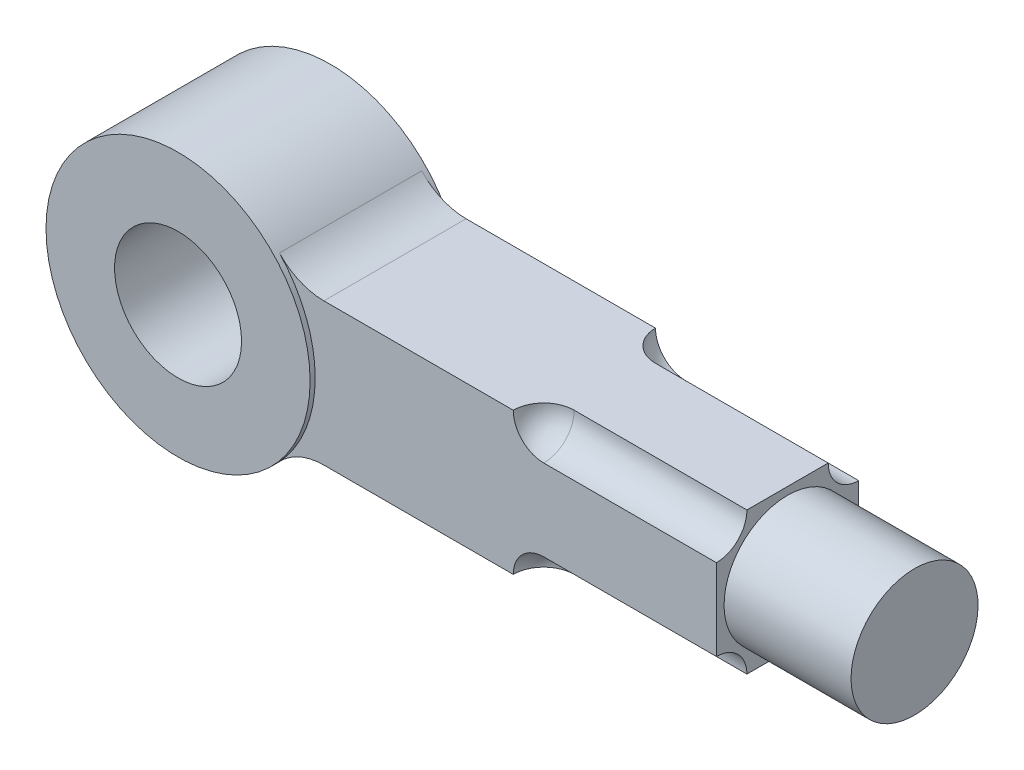
ISO-10303-21;
HEADER;
FILE_DESCRIPTION(('STEP AP214'),'2;1');
FILE_NAME('part.step','',(''),(''),'','','');
FILE_SCHEMA(('AUTOMOTIVE_DESIGN { 1 0 10303 214 1 1 1 1 }'));
ENDSEC;
DATA;
#1=APPLICATION_CONTEXT('core data for automotive mechanical design processes');
#2=APPLICATION_PROTOCOL_DEFINITION('international standard','automotive_design',2000,#1);
#3=PRODUCT_CONTEXT('',#1,'mechanical');
#4=PRODUCT('Part','Part','',(#3));
#5=PRODUCT_RELATED_PRODUCT_CATEGORY('part','',(#4));
#6=PRODUCT_DEFINITION_FORMATION('','',#4);
#7=PRODUCT_DEFINITION_CONTEXT('part definition',#1,'design');
#8=PRODUCT_DEFINITION('design','',#6,#7);
#9=PRODUCT_DEFINITION_SHAPE('','',#8);
#10=(LENGTH_UNIT() NAMED_UNIT(*) SI_UNIT(.MILLI.,.METRE.));
#11=(NAMED_UNIT(*) PLANE_ANGLE_UNIT() SI_UNIT($,.RADIAN.));
#12=(NAMED_UNIT(*) SI_UNIT($,.STERADIAN.) SOLID_ANGLE_UNIT());
#13=UNCERTAINTY_MEASURE_WITH_UNIT(LENGTH_MEASURE(1.E-05),#10,'distance_accuracy_value','');
#14=(GEOMETRIC_REPRESENTATION_CONTEXT(3) GLOBAL_UNCERTAINTY_ASSIGNED_CONTEXT((#13)) GLOBAL_UNIT_ASSIGNED_CONTEXT((#10,
#11,#12)) REPRESENTATION_CONTEXT('',''));
#15=CARTESIAN_POINT('',(0.,0.,0.));
#16=DIRECTION('',(0.,0.,1.));
#17=DIRECTION('',(1.,0.,0.));
#18=AXIS2_PLACEMENT_3D('',#15,#16,#17);
#19=CARTESIAN_POINT('',(0.,0.,15.));
#20=DIRECTION('',(0.,0.,1.));
#21=DIRECTION('',(1.,0.,0.));
#22=AXIS2_PLACEMENT_3D('',#19,#20,#21);
#23=PLANE('',#22);
#24=CARTESIAN_POINT('',(0.,0.,15.));
#25=DIRECTION('',(0.,0.,1.));
#26=DIRECTION('',(1.,0.,0.));
#27=AXIS2_PLACEMENT_3D('',#24,#25,#26);
#28=CIRCLE('',#27,26.);
#29=CARTESIAN_POINT('',(26.,0.,15.));
#30=VERTEX_POINT('',#29);
#31=EDGE_CURVE('E193',#30,#30,#28,.T.);
#32=ORIENTED_EDGE('',*,*,#31,.T.);
#33=EDGE_LOOP('',(#32));
#34=FACE_BOUND('',#33,.T.);
#35=CARTESIAN_POINT('',(0.,0.,15.));
#36=DIRECTION('',(0.,0.,1.));
#37=DIRECTION('',(1.,0.,0.));
#38=AXIS2_PLACEMENT_3D('',#35,#36,#37);
#39=CIRCLE('',#38,12.5);
#40=CARTESIAN_POINT('',(12.5,0.,15.));
#41=VERTEX_POINT('',#40);
#42=EDGE_CURVE('E186',#41,#41,#39,.T.);
#43=ORIENTED_EDGE('',*,*,#42,.F.);
#44=EDGE_LOOP('',(#43));
#45=FACE_BOUND('',#44,.T.);
#46=ADVANCED_FACE('F41',(#34,#45),#23,.T.);
#47=CARTESIAN_POINT('',(0.,0.,-15.));
#48=DIRECTION('',(0.,0.,1.));
#49=DIRECTION('',(1.,0.,0.));
#50=AXIS2_PLACEMENT_3D('',#47,#48,#49);
#51=PLANE('',#50);
#52=CARTESIAN_POINT('',(0.,0.,-15.));
#53=DIRECTION('',(0.,0.,1.));
#54=DIRECTION('',(1.,0.,0.));
#55=AXIS2_PLACEMENT_3D('',#52,#53,#54);
#56=CIRCLE('',#55,26.);
#57=CARTESIAN_POINT('',(26.,0.,-15.));
#58=VERTEX_POINT('',#57);
#59=EDGE_CURVE('E195',#58,#58,#56,.T.);
#60=ORIENTED_EDGE('',*,*,#59,.F.);
#61=EDGE_LOOP('',(#60));
#62=FACE_BOUND('',#61,.T.);
#63=CARTESIAN_POINT('',(0.,0.,-15.));
#64=DIRECTION('',(0.,0.,1.));
#65=DIRECTION('',(1.,0.,0.));
#66=AXIS2_PLACEMENT_3D('',#63,#64,#65);
#67=CIRCLE('',#66,12.5);
#68=CARTESIAN_POINT('',(12.5,0.,-15.));
#69=VERTEX_POINT('',#68);
#70=EDGE_CURVE('E189',#69,#69,#67,.T.);
#71=ORIENTED_EDGE('',*,*,#70,.T.);
#72=EDGE_LOOP('',(#71));
#73=FACE_BOUND('',#72,.T.);
#74=ADVANCED_FACE('F316',(#62,#73),#51,.F.);
#75=CARTESIAN_POINT('',(0.,0.,15.));
#76=DIRECTION('',(0.,0.,-1.));
#77=DIRECTION('',(-1.,0.,0.));
#78=AXIS2_PLACEMENT_3D('',#75,#76,#77);
#79=CYLINDRICAL_SURFACE('',#78,26.);
#80=CARTESIAN_POINT('',(0.,0.,-14.));
#81=DIRECTION('',(0.,0.,1.));
#82=DIRECTION('',(1.,0.,0.));
#83=AXIS2_PLACEMENT_3D('',#80,#81,#82);
#84=CIRCLE('',#83,26.);
#85=CARTESIAN_POINT('',(18.9613983144382,-17.7894736842105,-14.));
#86=VERTEX_POINT('',#85);
#87=CARTESIAN_POINT('',(18.9613983144382,17.7894736842105,-14.));
#88=VERTEX_POINT('',#87);
#89=EDGE_CURVE('E177',#86,#88,#84,.T.);
#90=ORIENTED_EDGE('',*,*,#89,.F.);
#91=DIRECTION('',(0.,0.,-1.));
#92=VECTOR('',#91,1.);
#93=CARTESIAN_POINT('',(18.9613983144382,-17.7894736842105,15.));
#94=LINE('',#93,#92);
#95=CARTESIAN_POINT('',(18.9613983144382,-17.7894736842105,14.));
#96=VERTEX_POINT('',#95);
#97=EDGE_CURVE('E207',#86,#96,#94,.F.);
#98=ORIENTED_EDGE('',*,*,#97,.T.);
#99=CARTESIAN_POINT('',(0.,0.,14.));
#100=DIRECTION('',(0.,0.,1.));
#101=DIRECTION('',(1.,0.,0.));
#102=AXIS2_PLACEMENT_3D('',#99,#100,#101);
#103=CIRCLE('',#102,26.);
#104=CARTESIAN_POINT('',(18.9613983144382,17.7894736842105,14.));
#105=VERTEX_POINT('',#104);
#106=EDGE_CURVE('E180',#96,#105,#103,.T.);
#107=ORIENTED_EDGE('',*,*,#106,.T.);
#108=DIRECTION('',(0.,0.,-1.));
#109=VECTOR('',#108,1.);
#110=CARTESIAN_POINT('',(18.9613983144382,17.7894736842105,15.));
#111=LINE('',#110,#109);
#112=EDGE_CURVE('E204',#105,#88,#111,.T.);
#113=ORIENTED_EDGE('',*,*,#112,.T.);
#114=EDGE_LOOP('',(#90,#98,#107,#113));
#115=FACE_BOUND('',#114,.T.);
#116=ORIENTED_EDGE('',*,*,#31,.F.);
#117=EDGE_LOOP('',(#116));
#118=FACE_BOUND('',#117,.T.);
#119=ORIENTED_EDGE('',*,*,#59,.T.);
#120=EDGE_LOOP('',(#119));
#121=FACE_BOUND('',#120,.T.);
#122=ADVANCED_FACE('F280',(#115,#118,#121),#79,.T.);
#123=CARTESIAN_POINT('',(0.,0.,15.));
#124=DIRECTION('',(0.,0.,-1.));
#125=DIRECTION('',(-1.,0.,0.));
#126=AXIS2_PLACEMENT_3D('',#123,#124,#125);
#127=CYLINDRICAL_SURFACE('',#126,12.5);
#128=ORIENTED_EDGE('',*,*,#42,.T.);
#129=EDGE_LOOP('',(#128));
#130=FACE_BOUND('',#129,.T.);
#131=ORIENTED_EDGE('',*,*,#70,.F.);
#132=EDGE_LOOP('',(#131));
#133=FACE_BOUND('',#132,.T.);
#134=ADVANCED_FACE('F317',(#130,#133),#127,.F.);
#135=CARTESIAN_POINT('',(0.,-14.,14.));
#136=DIRECTION('',(0.,-1.,0.));
#137=DIRECTION('',(1.,0.,0.));
#138=AXIS2_PLACEMENT_3D('',#135,#136,#137);
#139=PLANE('',#138);
#140=DIRECTION('',(1.,0.,0.));
#141=VECTOR('',#140,1.);
#142=CARTESIAN_POINT('',(65.,-14.,8.));
#143=LINE('',#142,#141);
#144=CARTESIAN_POINT('',(71.,-14.,8.));
#145=VERTEX_POINT('',#144);
#146=CARTESIAN_POINT('',(105.,-14.,8.));
#147=VERTEX_POINT('',#146);
#148=EDGE_CURVE('E254',#145,#147,#143,.T.);
#149=ORIENTED_EDGE('',*,*,#148,.F.);
#150=CARTESIAN_POINT('',(71.,-14.,14.));
#151=DIRECTION('',(0.,-1.,0.));
#152=DIRECTION('',(1.,0.,0.));
#153=AXIS2_PLACEMENT_3D('',#150,#151,#152);
#154=CIRCLE('',#153,6.);
#155=CARTESIAN_POINT('',(65.,-14.,14.));
#156=VERTEX_POINT('',#155);
#157=EDGE_CURVE('E44',#145,#156,#154,.F.);
#158=ORIENTED_EDGE('',*,*,#157,.T.);
#159=DIRECTION('',(-1.,0.,0.));
#160=VECTOR('',#159,1.);
#161=CARTESIAN_POINT('',(0.,-14.,14.));
#162=LINE('',#161,#160);
#163=CARTESIAN_POINT('',(27.712812921102,-14.,14.));
#164=VERTEX_POINT('',#163);
#165=EDGE_CURVE('E252',#156,#164,#162,.T.);
#166=ORIENTED_EDGE('',*,*,#165,.T.);
#167=DIRECTION('',(0.,0.,-1.));
#168=VECTOR('',#167,1.);
#169=CARTESIAN_POINT('',(27.712812921102,-14.,14.));
#170=LINE('',#169,#168);
#171=CARTESIAN_POINT('',(27.712812921102,-14.,-14.));
#172=VERTEX_POINT('',#171);
#173=EDGE_CURVE('E200',#164,#172,#170,.T.);
#174=ORIENTED_EDGE('',*,*,#173,.T.);
#175=DIRECTION('',(-1.,0.,0.));
#176=VECTOR('',#175,1.);
#177=CARTESIAN_POINT('',(0.,-14.,-14.));
#178=LINE('',#177,#176);
#179=CARTESIAN_POINT('',(65.,-14.,-14.));
#180=VERTEX_POINT('',#179);
#181=EDGE_CURVE('E174',#180,#172,#178,.T.);
#182=ORIENTED_EDGE('',*,*,#181,.F.);
#183=CARTESIAN_POINT('',(71.,-14.,-14.));
#184=DIRECTION('',(0.,-1.,0.));
#185=DIRECTION('',(1.,0.,0.));
#186=AXIS2_PLACEMENT_3D('',#183,#184,#185);
#187=CIRCLE('',#186,6.);
#188=CARTESIAN_POINT('',(71.,-14.,-8.));
#189=VERTEX_POINT('',#188);
#190=EDGE_CURVE('E243',#180,#189,#187,.F.);
#191=ORIENTED_EDGE('',*,*,#190,.T.);
#192=DIRECTION('',(1.,0.,0.));
#193=VECTOR('',#192,1.);
#194=CARTESIAN_POINT('',(65.,-14.,-8.));
#195=LINE('',#194,#193);
#196=CARTESIAN_POINT('',(105.,-14.,-8.));
#197=VERTEX_POINT('',#196);
#198=EDGE_CURVE('E271',#197,#189,#195,.F.);
#199=ORIENTED_EDGE('',*,*,#198,.F.);
#200=DIRECTION('',(0.,0.,-1.));
#201=VECTOR('',#200,1.);
#202=CARTESIAN_POINT('',(105.,-14.,14.));
#203=LINE('',#202,#201);
#204=EDGE_CURVE('E184',#147,#197,#203,.T.);
#205=ORIENTED_EDGE('',*,*,#204,.F.);
#206=EDGE_LOOP('',(#149,#158,#166,#174,#182,#191,#199,#205));
#207=FACE_BOUND('',#206,.T.);
#208=ADVANCED_FACE('F249',(#207),#139,.T.);
#209=CARTESIAN_POINT('',(105.,0.,14.));
#210=DIRECTION('',(1.,0.,0.));
#211=DIRECTION('',(0.,1.,0.));
#212=AXIS2_PLACEMENT_3D('',#209,#210,#211);
#213=PLANE('',#212);
#214=CARTESIAN_POINT('',(105.,0.,0.));
#215=DIRECTION('',(1.,0.,0.));
#216=DIRECTION('',(0.,1.,0.));
#217=AXIS2_PLACEMENT_3D('',#214,#215,#216);
#218=CIRCLE('',#217,12.5);
#219=CARTESIAN_POINT('',(105.,12.5000000000001,0.));
#220=VERTEX_POINT('',#219);
#221=EDGE_CURVE('E11',#220,#220,#218,.T.);
#222=ORIENTED_EDGE('',*,*,#221,.F.);
#223=EDGE_LOOP('',(#222));
#224=FACE_BOUND('',#223,.T.);
#225=CARTESIAN_POINT('',(105.,-13.9999999999999,14.));
#226=DIRECTION('',(1.,0.,0.));
#227=DIRECTION('',(0.,-1.,0.));
#228=AXIS2_PLACEMENT_3D('',#225,#226,#227);
#229=CIRCLE('',#228,6.);
#230=CARTESIAN_POINT('',(105.,-7.9999999999999,14.));
#231=VERTEX_POINT('',#230);
#232=EDGE_CURVE('E264',#147,#231,#229,.T.);
#233=ORIENTED_EDGE('',*,*,#232,.F.);
#234=ORIENTED_EDGE('',*,*,#204,.T.);
#235=CARTESIAN_POINT('',(105.,-13.9999999999999,-14.));
#236=DIRECTION('',(1.,0.,0.));
#237=DIRECTION('',(0.,1.,0.));
#238=AXIS2_PLACEMENT_3D('',#235,#236,#237);
#239=CIRCLE('',#238,6.);
#240=CARTESIAN_POINT('',(105.,-7.9999999999999,-14.));
#241=VERTEX_POINT('',#240);
#242=EDGE_CURVE('E166',#241,#197,#239,.T.);
#243=ORIENTED_EDGE('',*,*,#242,.F.);
#244=DIRECTION('',(0.,-1.,0.));
#245=VECTOR('',#244,1.);
#246=CARTESIAN_POINT('',(105.,0.,-14.));
#247=LINE('',#246,#245);
#248=CARTESIAN_POINT('',(105.,8.00000000000001,-14.));
#249=VERTEX_POINT('',#248);
#250=EDGE_CURVE('E146',#249,#241,#247,.T.);
#251=ORIENTED_EDGE('',*,*,#250,.F.);
#252=CARTESIAN_POINT('',(105.,14.,-14.));
#253=DIRECTION('',(1.,0.,0.));
#254=DIRECTION('',(0.,-1.,0.));
#255=AXIS2_PLACEMENT_3D('',#252,#253,#254);
#256=CIRCLE('',#255,6.);
#257=CARTESIAN_POINT('',(105.,14.,-8.));
#258=VERTEX_POINT('',#257);
#259=EDGE_CURVE('E160',#258,#249,#256,.T.);
#260=ORIENTED_EDGE('',*,*,#259,.F.);
#261=DIRECTION('',(0.,0.,-1.));
#262=VECTOR('',#261,1.);
#263=CARTESIAN_POINT('',(105.,14.,14.));
#264=LINE('',#263,#262);
#265=CARTESIAN_POINT('',(105.,14.,8.));
#266=VERTEX_POINT('',#265);
#267=EDGE_CURVE('E182',#266,#258,#264,.T.);
#268=ORIENTED_EDGE('',*,*,#267,.F.);
#269=CARTESIAN_POINT('',(105.,14.,14.));
#270=DIRECTION('',(1.,0.,0.));
#271=DIRECTION('',(0.,1.,0.));
#272=AXIS2_PLACEMENT_3D('',#269,#270,#271);
#273=CIRCLE('',#272,6.);
#274=CARTESIAN_POINT('',(105.,8.,14.));
#275=VERTEX_POINT('',#274);
#276=EDGE_CURVE('E170',#275,#266,#273,.T.);
#277=ORIENTED_EDGE('',*,*,#276,.F.);
#278=DIRECTION('',(0.,-1.,0.));
#279=VECTOR('',#278,1.);
#280=CARTESIAN_POINT('',(105.,0.,14.));
#281=LINE('',#280,#279);
#282=EDGE_CURVE('E260',#275,#231,#281,.T.);
#283=ORIENTED_EDGE('',*,*,#282,.T.);
#284=EDGE_LOOP('',(#233,#234,#243,#251,#260,#268,#277,#283));
#285=FACE_BOUND('',#284,.T.);
#286=ADVANCED_FACE('F175',(#224,#285),#213,.T.);
#287=CARTESIAN_POINT('',(0.,14.,14.));
#288=DIRECTION('',(0.,-1.,0.));
#289=DIRECTION('',(1.,0.,0.));
#290=AXIS2_PLACEMENT_3D('',#287,#288,#289);
#291=PLANE('',#290);
#292=ORIENTED_EDGE('',*,*,#267,.T.);
#293=DIRECTION('',(1.,0.,0.));
#294=VECTOR('',#293,1.);
#295=CARTESIAN_POINT('',(65.,14.,-8.));
#296=LINE('',#295,#294);
#297=CARTESIAN_POINT('',(71.,14.,-8.));
#298=VERTEX_POINT('',#297);
#299=EDGE_CURVE('E161',#258,#298,#296,.F.);
#300=ORIENTED_EDGE('',*,*,#299,.T.);
#301=CARTESIAN_POINT('',(71.,14.,-14.));
#302=DIRECTION('',(0.,-1.,0.));
#303=DIRECTION('',(1.,0.,0.));
#304=AXIS2_PLACEMENT_3D('',#301,#302,#303);
#305=CIRCLE('',#304,6.);
#306=CARTESIAN_POINT('',(65.,14.,-14.));
#307=VERTEX_POINT('',#306);
#308=EDGE_CURVE('E233',#298,#307,#305,.T.);
#309=ORIENTED_EDGE('',*,*,#308,.T.);
#310=DIRECTION('',(-1.,0.,0.));
#311=VECTOR('',#310,1.);
#312=CARTESIAN_POINT('',(0.,14.,-14.));
#313=LINE('',#312,#311);
#314=CARTESIAN_POINT('',(27.712812921102,14.,-14.));
#315=VERTEX_POINT('',#314);
#316=EDGE_CURVE('E172',#307,#315,#313,.T.);
#317=ORIENTED_EDGE('',*,*,#316,.T.);
#318=DIRECTION('',(0.,0.,1.));
#319=VECTOR('',#318,1.);
#320=CARTESIAN_POINT('',(27.712812921102,14.,14.));
#321=LINE('',#320,#319);
#322=CARTESIAN_POINT('',(27.712812921102,14.,14.));
#323=VERTEX_POINT('',#322);
#324=EDGE_CURVE('E209',#315,#323,#321,.T.);
#325=ORIENTED_EDGE('',*,*,#324,.T.);
#326=DIRECTION('',(-1.,0.,0.));
#327=VECTOR('',#326,1.);
#328=CARTESIAN_POINT('',(0.,14.,14.));
#329=LINE('',#328,#327);
#330=CARTESIAN_POINT('',(65.,14.,14.));
#331=VERTEX_POINT('',#330);
#332=EDGE_CURVE('E187',#331,#323,#329,.T.);
#333=ORIENTED_EDGE('',*,*,#332,.F.);
#334=CARTESIAN_POINT('',(71.,14.,14.));
#335=DIRECTION('',(0.,-1.,0.));
#336=DIRECTION('',(1.,0.,0.));
#337=AXIS2_PLACEMENT_3D('',#334,#335,#336);
#338=CIRCLE('',#337,6.);
#339=CARTESIAN_POINT('',(71.,14.,8.));
#340=VERTEX_POINT('',#339);
#341=EDGE_CURVE('E236',#331,#340,#338,.T.);
#342=ORIENTED_EDGE('',*,*,#341,.T.);
#343=DIRECTION('',(1.,0.,0.));
#344=VECTOR('',#343,1.);
#345=CARTESIAN_POINT('',(65.,14.,8.));
#346=LINE('',#345,#344);
#347=EDGE_CURVE('E272',#340,#266,#346,.T.);
#348=ORIENTED_EDGE('',*,*,#347,.T.);
#349=EDGE_LOOP('',(#292,#300,#309,#317,#325,#333,#342,#348));
#350=FACE_BOUND('',#349,.T.);
#351=ADVANCED_FACE('F288',(#350),#291,.F.);
#352=CARTESIAN_POINT('',(0.,0.,14.));
#353=DIRECTION('',(0.,0.,1.));
#354=DIRECTION('',(1.,0.,0.));
#355=AXIS2_PLACEMENT_3D('',#352,#353,#354);
#356=PLANE('',#355);
#357=DIRECTION('',(1.,0.,0.));
#358=VECTOR('',#357,1.);
#359=CARTESIAN_POINT('',(65.,-7.99999999999991,14.));
#360=LINE('',#359,#358);
#361=CARTESIAN_POINT('',(71.,-7.99999999999991,14.));
#362=VERTEX_POINT('',#361);
#363=EDGE_CURVE('E228',#231,#362,#360,.F.);
#364=ORIENTED_EDGE('',*,*,#363,.F.);
#365=ORIENTED_EDGE('',*,*,#282,.F.);
#366=DIRECTION('',(1.,0.,0.));
#367=VECTOR('',#366,1.);
#368=CARTESIAN_POINT('',(65.,7.99999999999998,14.));
#369=LINE('',#368,#367);
#370=CARTESIAN_POINT('',(71.,7.99999999999998,14.));
#371=VERTEX_POINT('',#370);
#372=EDGE_CURVE('E223',#371,#275,#369,.T.);
#373=ORIENTED_EDGE('',*,*,#372,.F.);
#374=CARTESIAN_POINT('',(71.,14.,14.));
#375=DIRECTION('',(0.,0.,1.));
#376=DIRECTION('',(1.,0.,0.));
#377=AXIS2_PLACEMENT_3D('',#374,#375,#376);
#378=CIRCLE('',#377,6.);
#379=EDGE_CURVE('E238',#371,#331,#378,.F.);
#380=ORIENTED_EDGE('',*,*,#379,.T.);
#381=ORIENTED_EDGE('',*,*,#332,.T.);
#382=CARTESIAN_POINT('',(27.712812921102,26.,14.));
#383=DIRECTION('',(0.,0.,1.));
#384=DIRECTION('',(1.,0.,0.));
#385=AXIS2_PLACEMENT_3D('',#382,#383,#384);
#386=CIRCLE('',#385,12.);
#387=EDGE_CURVE('E157',#323,#105,#386,.F.);
#388=ORIENTED_EDGE('',*,*,#387,.T.);
#389=ORIENTED_EDGE('',*,*,#106,.F.);
#390=CARTESIAN_POINT('',(27.712812921102,-26.,14.));
#391=DIRECTION('',(0.,0.,1.));
#392=DIRECTION('',(1.,0.,0.));
#393=AXIS2_PLACEMENT_3D('',#390,#391,#392);
#394=CIRCLE('',#393,12.);
#395=EDGE_CURVE('E213',#96,#164,#394,.F.);
#396=ORIENTED_EDGE('',*,*,#395,.T.);
#397=ORIENTED_EDGE('',*,*,#165,.F.);
#398=CARTESIAN_POINT('',(71.,-13.9999999999999,14.));
#399=DIRECTION('',(0.,0.,1.));
#400=DIRECTION('',(1.,0.,0.));
#401=AXIS2_PLACEMENT_3D('',#398,#399,#400);
#402=CIRCLE('',#401,6.);
#403=EDGE_CURVE('E60',#156,#362,#402,.F.);
#404=ORIENTED_EDGE('',*,*,#403,.T.);
#405=EDGE_LOOP('',(#364,#365,#373,#380,#381,#388,#389,#396,#397,#404));
#406=FACE_BOUND('',#405,.T.);
#407=ADVANCED_FACE('F251',(#406),#356,.T.);
#408=CARTESIAN_POINT('',(0.,0.,-14.));
#409=DIRECTION('',(0.,0.,1.));
#410=DIRECTION('',(1.,0.,0.));
#411=AXIS2_PLACEMENT_3D('',#408,#409,#410);
#412=PLANE('',#411);
#413=ORIENTED_EDGE('',*,*,#250,.T.);
#414=DIRECTION('',(1.,0.,0.));
#415=VECTOR('',#414,1.);
#416=CARTESIAN_POINT('',(65.,-7.99999999999992,-14.));
#417=LINE('',#416,#415);
#418=CARTESIAN_POINT('',(71.,-7.99999999999992,-14.));
#419=VERTEX_POINT('',#418);
#420=EDGE_CURVE('E156',#241,#419,#417,.F.);
#421=ORIENTED_EDGE('',*,*,#420,.T.);
#422=CARTESIAN_POINT('',(71.,-13.9999999999999,-14.));
#423=DIRECTION('',(0.,0.,1.));
#424=DIRECTION('',(1.,0.,0.));
#425=AXIS2_PLACEMENT_3D('',#422,#423,#424);
#426=CIRCLE('',#425,6.);
#427=EDGE_CURVE('E244',#419,#180,#426,.T.);
#428=ORIENTED_EDGE('',*,*,#427,.T.);
#429=ORIENTED_EDGE('',*,*,#181,.T.);
#430=CARTESIAN_POINT('',(27.712812921102,-26.,-14.));
#431=DIRECTION('',(0.,0.,1.));
#432=DIRECTION('',(1.,0.,0.));
#433=AXIS2_PLACEMENT_3D('',#430,#431,#432);
#434=CIRCLE('',#433,12.);
#435=EDGE_CURVE('E215',#172,#86,#434,.T.);
#436=ORIENTED_EDGE('',*,*,#435,.T.);
#437=ORIENTED_EDGE('',*,*,#89,.T.);
#438=CARTESIAN_POINT('',(27.712812921102,26.,-14.));
#439=DIRECTION('',(0.,0.,1.));
#440=DIRECTION('',(1.,0.,0.));
#441=AXIS2_PLACEMENT_3D('',#438,#439,#440);
#442=CIRCLE('',#441,12.);
#443=EDGE_CURVE('E220',#88,#315,#442,.T.);
#444=ORIENTED_EDGE('',*,*,#443,.T.);
#445=ORIENTED_EDGE('',*,*,#316,.F.);
#446=CARTESIAN_POINT('',(71.,14.,-14.));
#447=DIRECTION('',(0.,0.,1.));
#448=DIRECTION('',(1.,0.,0.));
#449=AXIS2_PLACEMENT_3D('',#446,#447,#448);
#450=CIRCLE('',#449,6.);
#451=CARTESIAN_POINT('',(71.,7.99999999999999,-14.));
#452=VERTEX_POINT('',#451);
#453=EDGE_CURVE('E151',#307,#452,#450,.T.);
#454=ORIENTED_EDGE('',*,*,#453,.T.);
#455=DIRECTION('',(1.,0.,0.));
#456=VECTOR('',#455,1.);
#457=CARTESIAN_POINT('',(65.,7.99999999999999,-14.));
#458=LINE('',#457,#456);
#459=EDGE_CURVE('E144',#452,#249,#458,.T.);
#460=ORIENTED_EDGE('',*,*,#459,.T.);
#461=EDGE_LOOP('',(#413,#421,#428,#429,#436,#437,#444,#445,#454,#460));
#462=FACE_BOUND('',#461,.T.);
#463=ADVANCED_FACE('F147',(#462),#412,.F.);
#464=CARTESIAN_POINT('',(27.712812921102,-26.,15.));
#465=DIRECTION('',(0.,0.,-1.));
#466=DIRECTION('',(-1.,0.,0.));
#467=AXIS2_PLACEMENT_3D('',#464,#465,#466);
#468=CYLINDRICAL_SURFACE('',#467,12.);
#469=ORIENTED_EDGE('',*,*,#395,.F.);
#470=ORIENTED_EDGE('',*,*,#97,.F.);
#471=ORIENTED_EDGE('',*,*,#435,.F.);
#472=ORIENTED_EDGE('',*,*,#173,.F.);
#473=EDGE_LOOP('',(#469,#470,#471,#472));
#474=FACE_BOUND('',#473,.T.);
#475=ADVANCED_FACE('F332',(#474),#468,.F.);
#476=CARTESIAN_POINT('',(27.712812921102,26.,15.));
#477=DIRECTION('',(0.,0.,-1.));
#478=DIRECTION('',(-1.,0.,0.));
#479=AXIS2_PLACEMENT_3D('',#476,#477,#478);
#480=CYLINDRICAL_SURFACE('',#479,12.);
#481=ORIENTED_EDGE('',*,*,#387,.F.);
#482=ORIENTED_EDGE('',*,*,#324,.F.);
#483=ORIENTED_EDGE('',*,*,#443,.F.);
#484=ORIENTED_EDGE('',*,*,#112,.F.);
#485=EDGE_LOOP('',(#481,#482,#483,#484));
#486=FACE_BOUND('',#485,.T.);
#487=ADVANCED_FACE('F282',(#486),#480,.F.);
#488=CARTESIAN_POINT('',(65.,14.,-14.));
#489=DIRECTION('',(1.,0.,0.));
#490=DIRECTION('',(0.,1.,0.));
#491=AXIS2_PLACEMENT_3D('',#488,#489,#490);
#492=CYLINDRICAL_SURFACE('',#491,6.);
#493=ORIENTED_EDGE('',*,*,#459,.F.);
#494=CARTESIAN_POINT('',(71.,14.,-14.));
#495=DIRECTION('',(1.,0.,0.));
#496=DIRECTION('',(0.,1.,0.));
#497=AXIS2_PLACEMENT_3D('',#494,#495,#496);
#498=CIRCLE('',#497,6.);
#499=EDGE_CURVE('E226',#452,#298,#498,.F.);
#500=ORIENTED_EDGE('',*,*,#499,.T.);
#501=ORIENTED_EDGE('',*,*,#299,.F.);
#502=ORIENTED_EDGE('',*,*,#259,.T.);
#503=EDGE_LOOP('',(#493,#500,#501,#502));
#504=FACE_BOUND('',#503,.T.);
#505=ADVANCED_FACE('F163',(#504),#492,.F.);
#506=CARTESIAN_POINT('',(65.,-13.9999999999999,-14.));
#507=DIRECTION('',(1.,0.,0.));
#508=DIRECTION('',(0.,1.,0.));
#509=AXIS2_PLACEMENT_3D('',#506,#507,#508);
#510=CYLINDRICAL_SURFACE('',#509,6.);
#511=ORIENTED_EDGE('',*,*,#198,.T.);
#512=CARTESIAN_POINT('',(71.,-13.9999999999999,-14.));
#513=DIRECTION('',(1.,0.,0.));
#514=DIRECTION('',(0.,1.,0.));
#515=AXIS2_PLACEMENT_3D('',#512,#513,#514);
#516=CIRCLE('',#515,6.);
#517=EDGE_CURVE('E239',#189,#419,#516,.F.);
#518=ORIENTED_EDGE('',*,*,#517,.T.);
#519=ORIENTED_EDGE('',*,*,#420,.F.);
#520=ORIENTED_EDGE('',*,*,#242,.T.);
#521=EDGE_LOOP('',(#511,#518,#519,#520));
#522=FACE_BOUND('',#521,.T.);
#523=ADVANCED_FACE('F354',(#522),#510,.F.);
#524=CARTESIAN_POINT('',(65.,14.,14.));
#525=DIRECTION('',(1.,0.,0.));
#526=DIRECTION('',(0.,1.,0.));
#527=AXIS2_PLACEMENT_3D('',#524,#525,#526);
#528=CYLINDRICAL_SURFACE('',#527,6.);
#529=ORIENTED_EDGE('',*,*,#347,.F.);
#530=CARTESIAN_POINT('',(71.,14.,14.));
#531=DIRECTION('',(1.,0.,0.));
#532=DIRECTION('',(0.,1.,0.));
#533=AXIS2_PLACEMENT_3D('',#530,#531,#532);
#534=CIRCLE('',#533,6.);
#535=EDGE_CURVE('E231',#340,#371,#534,.F.);
#536=ORIENTED_EDGE('',*,*,#535,.T.);
#537=ORIENTED_EDGE('',*,*,#372,.T.);
#538=ORIENTED_EDGE('',*,*,#276,.T.);
#539=EDGE_LOOP('',(#529,#536,#537,#538));
#540=FACE_BOUND('',#539,.T.);
#541=ADVANCED_FACE('F358',(#540),#528,.F.);
#542=CARTESIAN_POINT('',(65.,-13.9999999999999,14.));
#543=DIRECTION('',(1.,0.,0.));
#544=DIRECTION('',(0.,1.,0.));
#545=AXIS2_PLACEMENT_3D('',#542,#543,#544);
#546=CYLINDRICAL_SURFACE('',#545,6.);
#547=ORIENTED_EDGE('',*,*,#363,.T.);
#548=CARTESIAN_POINT('',(71.,-13.9999999999999,14.));
#549=DIRECTION('',(1.,0.,0.));
#550=DIRECTION('',(0.,1.,0.));
#551=AXIS2_PLACEMENT_3D('',#548,#549,#550);
#552=CIRCLE('',#551,6.);
#553=EDGE_CURVE('E250',#362,#145,#552,.F.);
#554=ORIENTED_EDGE('',*,*,#553,.T.);
#555=ORIENTED_EDGE('',*,*,#148,.T.);
#556=ORIENTED_EDGE('',*,*,#232,.T.);
#557=EDGE_LOOP('',(#547,#554,#555,#556));
#558=FACE_BOUND('',#557,.T.);
#559=ADVANCED_FACE('F258',(#558),#546,.F.);
#560=CARTESIAN_POINT('',(71.,14.,-14.));
#561=DIRECTION('',(-1.,0.,0.));
#562=DIRECTION('',(0.,-1.,0.));
#563=AXIS2_PLACEMENT_3D('',#560,#561,#562);
#564=SPHERICAL_SURFACE('',#563,6.);
#565=ORIENTED_EDGE('',*,*,#308,.F.);
#566=ORIENTED_EDGE('',*,*,#499,.F.);
#567=ORIENTED_EDGE('',*,*,#453,.F.);
#568=EDGE_LOOP('',(#565,#566,#567));
#569=FACE_BOUND('',#568,.T.);
#570=ADVANCED_FACE('F289',(#569),#564,.F.);
#571=CARTESIAN_POINT('',(71.,14.,14.));
#572=DIRECTION('',(1.,0.,0.));
#573=DIRECTION('',(0.,1.,0.));
#574=AXIS2_PLACEMENT_3D('',#571,#572,#573);
#575=SPHERICAL_SURFACE('',#574,6.);
#576=ORIENTED_EDGE('',*,*,#379,.F.);
#577=ORIENTED_EDGE('',*,*,#535,.F.);
#578=ORIENTED_EDGE('',*,*,#341,.F.);
#579=EDGE_LOOP('',(#576,#577,#578));
#580=FACE_BOUND('',#579,.T.);
#581=ADVANCED_FACE('F338',(#580),#575,.F.);
#582=CARTESIAN_POINT('',(71.,-13.9999999999999,-14.));
#583=DIRECTION('',(1.,0.,0.));
#584=DIRECTION('',(0.,1.,0.));
#585=AXIS2_PLACEMENT_3D('',#582,#583,#584);
#586=SPHERICAL_SURFACE('',#585,6.);
#587=ORIENTED_EDGE('',*,*,#427,.F.);
#588=ORIENTED_EDGE('',*,*,#517,.F.);
#589=ORIENTED_EDGE('',*,*,#190,.F.);
#590=EDGE_LOOP('',(#587,#588,#589));
#591=FACE_BOUND('',#590,.T.);
#592=ADVANCED_FACE('F345',(#591),#586,.F.);
#593=CARTESIAN_POINT('',(71.,-13.9999999999999,14.));
#594=DIRECTION('',(-1.,0.,0.));
#595=DIRECTION('',(0.,-1.,0.));
#596=AXIS2_PLACEMENT_3D('',#593,#594,#595);
#597=SPHERICAL_SURFACE('',#596,6.);
#598=ORIENTED_EDGE('',*,*,#157,.F.);
#599=ORIENTED_EDGE('',*,*,#553,.F.);
#600=ORIENTED_EDGE('',*,*,#403,.F.);
#601=EDGE_LOOP('',(#598,#599,#600));
#602=FACE_BOUND('',#601,.T.);
#603=ADVANCED_FACE('F43',(#602),#597,.F.);
#604=CARTESIAN_POINT('',(130.,0.,0.));
#605=DIRECTION('',(-1.,0.,0.));
#606=DIRECTION('',(0.,-1.,0.));
#607=AXIS2_PLACEMENT_3D('',#604,#605,#606);
#608=CYLINDRICAL_SURFACE('',#607,12.5);
#609=CARTESIAN_POINT('',(130.,0.,0.));
#610=DIRECTION('',(1.,0.,0.));
#611=DIRECTION('',(0.,1.,0.));
#612=AXIS2_PLACEMENT_3D('',#609,#610,#611);
#613=CIRCLE('',#612,12.5);
#614=CARTESIAN_POINT('',(130.,12.5000000000001,0.));
#615=VERTEX_POINT('',#614);
#616=EDGE_CURVE('E294',#615,#615,#613,.T.);
#617=ORIENTED_EDGE('',*,*,#616,.F.);
#618=EDGE_LOOP('',(#617));
#619=FACE_BOUND('',#618,.T.);
#620=ORIENTED_EDGE('',*,*,#221,.T.);
#621=EDGE_LOOP('',(#620));
#622=FACE_BOUND('',#621,.T.);
#623=ADVANCED_FACE('F305',(#619,#622),#608,.T.);
#624=CARTESIAN_POINT('',(130.,0.,0.));
#625=DIRECTION('',(1.,0.,0.));
#626=DIRECTION('',(0.,1.,0.));
#627=AXIS2_PLACEMENT_3D('',#624,#625,#626);
#628=PLANE('',#627);
#629=ORIENTED_EDGE('',*,*,#616,.T.);
#630=EDGE_LOOP('',(#629));
#631=FACE_BOUND('',#630,.T.);
#632=ADVANCED_FACE('F297',(#631),#628,.T.);
#633=CLOSED_SHELL('',(#46,#74,#122,#134,#208,#286,#351,#407,#463,#475,#487,#505,#523,#541,#559,
#570,#581,#592,#603,#623,#632));
#634=MANIFOLD_SOLID_BREP('B2',#633);
#635=ADVANCED_BREP_SHAPE_REPRESENTATION('',(#18,#634),#14);
#636=SHAPE_DEFINITION_REPRESENTATION(#9,#635);
ENDSEC;
END-ISO-10303-21;
